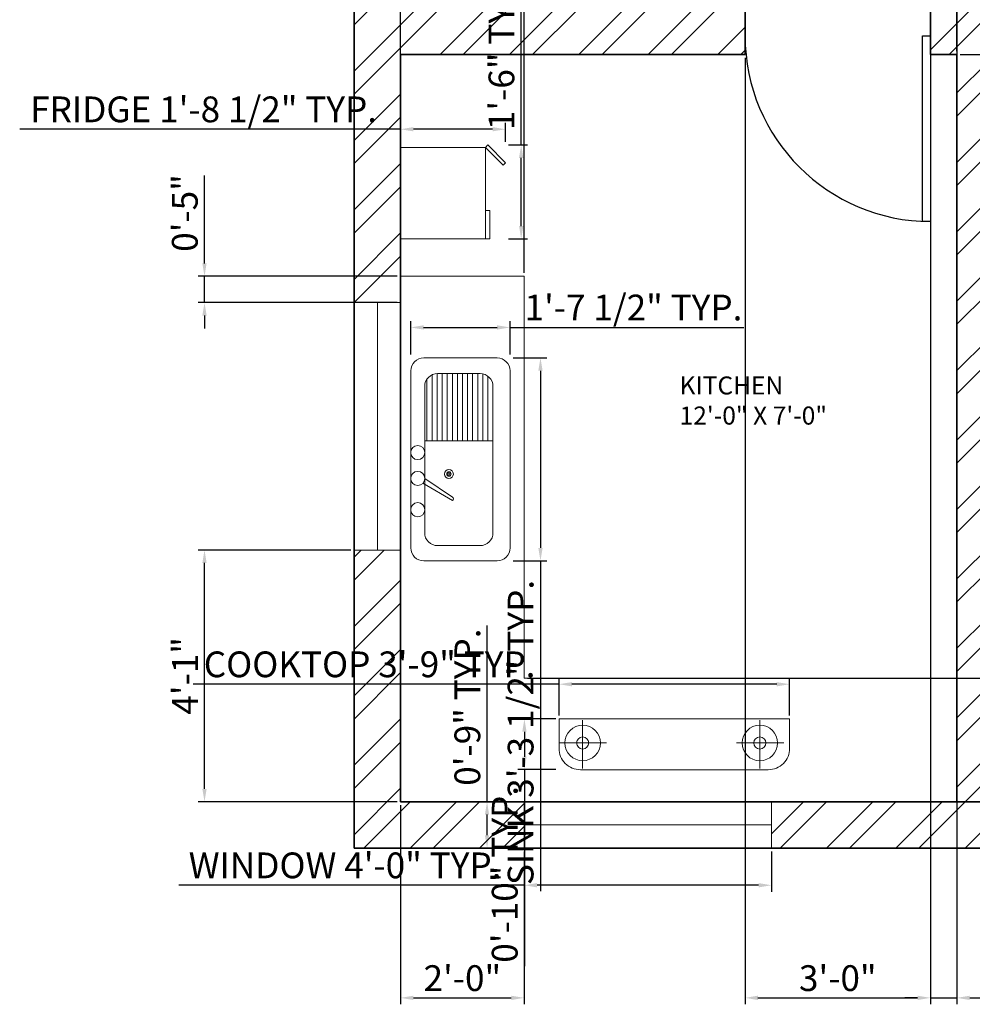
# Model space of a CAD drawing. Units: inches. Extents: x 28986 to 29505, y -162 to 451.
# Tile 1 of 6: x 28986 to 29171, y -159 to 32. Entities that reach past the tile are written whole.
import ezdxf

# ---------------------------------------------------------------- set-up
doc = ezdxf.new("R2010")
doc.units = ezdxf.units.IN
doc.layers.get('Defpoints').update_dxf_attribs({"color": 120})
doc.layers.add('A-ANNO-DIMS', color=9, linetype='Continuous', lineweight=18, true_color=0xafd9aa)
doc.layers.add('A-FLOR-CASE', color=32, linetype='Continuous', lineweight=18, true_color=0xcd6928)
for name, color, linetype, lineweight in [('A-AREA-IDEN', 6, 'Continuous', 18), ('A-EQPM', 8, 'Continuous', 18), ('A-FLOR-FIXT', 9, 'Continuous', 18), ('A-GLAZ', 4, 'Continuous', 18), ('A-WALL', 7, 'Continuous', 35), ('A-WALL-PATT', 1, 'Continuous', 13), ('DOOR', 2, 'Continuous', 25)]:
    doc.layers.add(name, color=color, linetype=linetype, lineweight=lineweight)
doc.styles.get("Standard").update_dxf_attribs({"font": 'arial.ttf'})
doc.dimstyles.new('ISO-25', dxfattribs={"dimtxt": 5, "dimasz": 2.5, "dimexe": 1.25, "dimexo": 0.625, "dimtad": 1, "dimdec": 0, "dimlunit": 3, "dimtxsty": 'Standard', "dimcen": 2.5, "dimadec": 0, "dimazin": 0, "dimtfac": 1, "dimtdec": 0, "dimtmove": 0, "dimatfit": 3, "dimfxl": 1, "dimarcsym": 0})

# ---------------------------------------------------------------- blocks, each defined once
blk = doc.blocks.new('*U7')
for p, q in [((-40, 0), (-40, 6)), ((0, 0), (0, 6))]:
    blk.add_line(p, q)
blk.add_lwpolyline([(0, 0), (0, -40), (-1.75, -40), (-1.75, 0)], close=True)
blk.add_arc((0, 0), 40, 180, 270)
blk = doc.blocks.new('FRIDGE')
for points in [[(0, 16.47), (17.77, 16.47), (17.77, 0), (0, 0)], [(0, 0), (5.53, 0), (5.53, -0.88), (0, -0.88)], [(18.23, -0.47), (17.77, 0), (14.32, -3.43), (14.79, -3.9)]]:
    blk.add_lwpolyline(points, close=True)
blk = doc.blocks.new('sink')
for p, q in [((-11.38, 27.19), (-5.63, 30.57)), ((-11.01, 26.26), (-5.62, 29.92)), ((-11.03, 19), (2.23, 19)), ((-10.58, 19), (-10.58, 7)), ((-9.6, 19), (-9.6, 6.16)), ((-8.61, 19), (-8.61, 5.92)), ((-7.63, 19), (-7.63, 5.92)), ((-6.64, 19), (-6.64, 5.92)), ((-5.66, 19), (-5.66, 5.92)), ((-4.67, 19), (-4.67, 5.92)), ((-3.69, 19), (-3.69, 5.92)), ((-2.7, 19), (-2.7, 5.92)), ((-1.72, 19), (-1.72, 5.92)), ((-0.73, 19), (-0.73, 5.92)), ((0.25, 19), (0.25, 5.98)), ((1.23, 19), (1.23, 6.43))]:
    blk.add_line(p, q)
for points in [[(-11.21, 42.26), (3.04, 42.26, -0.414214), (5.54, 39.76), (5.54, 5.38, -0.414214), (3.04, 2.88), (-11.21, 2.88, -0.414214), (-13.71, 5.38), (-13.71, 39.76, -0.414214)], [(-8.53, 39.31), (-0.27, 39.31, -0.414214), (2.23, 36.81), (2.23, 8.42, -0.414214), (-0.27, 5.92), (-8.53, 5.92, -0.414214), (-11.03, 8.42), (-11.03, 36.81, -0.414214)]]:
    blk.add_lwpolyline(points, format="xyb", close=True)
for centre, radius in [((-12.38, 32.33), 1.37), ((-12.38, 26.26), 1.37), ((-6.32, 25.41), 0.854), ((-6.32, 25.41), 0.432), ((-6.32, 25.41), 0.203), ((-12.38, 21.24), 1.37)]:
    blk.add_circle(centre, radius)
blk.add_arc((-5.86, 30.24), 0.398, 306.1138, 55.3114)
blk = doc.blocks.new('STOVE')
for p, q in [((-46.84, 5.62), (-46.82, 11.55)), ((-5.51, 5.62), (-5.49, 11.55)), ((-46.84, 5.62), (-52.42, 5.62)), ((-46.84, 5.62), (-46.84, 0.29)), ((-46.84, 5.62), (-41.4, 5.62)), ((-5.51, 5.62), (-11.1, 5.62)), ((-5.51, 5.62), (-5.51, 0.29)), ((-5.51, 5.62), (-0.08, 5.62))]:
    blk.add_line(p, q)
blk.add_lwpolyline([(-48.78, 11.85), (-5, 11.85, -0.414214), (0, 6.85), (0, 0), (-53.78, 0), (-53.78, 6.85, -0.414214)], format="xyb", close=True)
for centre, radius in [((-46.84, 5.62), 4.14), ((-5.51, 5.62), 4.14), ((-46.84, 5.62), 1.41), ((-5.51, 5.62), 1.41)]:
    blk.add_circle(centre, radius)
blk = doc.blocks.new('WIN-48IN')
for p, q in [((9, 48), (0, 48)), ((4.5, 0), (4.5, 48)), ((9, 0), (0, 0))]:
    blk.add_line(p, q)
blk = doc.blocks.new('*D37')
at = {"layer": 'A-ANNO-DIMS', "color": 0, "lineweight": -2, "transparency": 16777216}
for p, q in [((29084.16, -128.93), (29084.16, -136.75)), ((29132.16, -128.93), (29132.16, -136.75)), ((29084.16, -135.5), (29017.14, -135.5)), ((29129.66, -135.5), (29086.66, -135.5))]:
    blk.add_line(p, q, dxfattribs=at)
at = {"layer": 'A-ANNO-DIMS', "color": 0, "transparency": 16777216}
for points in [[(29086.66, -135.08), (29086.66, -135.92), (29084.16, -135.5)], [(29129.66, -135.08), (29129.66, -135.92), (29132.16, -135.5)]]:
    blk.add_solid(points, dxfattribs=at)
at = {"layer": 'Defpoints', "color": 0, "transparency": 16777216}
for p in [(29084.16, -128.3), (29132.16, -128.3), (29084.16, -135.5)]:
    blk.add_point(p, dxfattribs=at)
at = {"layer": 'A-ANNO-DIMS', "color": 0, "transparency": 16777216, "insert": (29049.4, -132.29), "char_height": 5, "attachment_point": 5}
blk.add_mtext('WINDOW 4\'-0" TYP.', dxfattribs=at)
blk = doc.blocks.new('*D38')
at = {"layer": 'A-ANNO-DIMS', "color": 0, "lineweight": -2, "transparency": 16777216}
for p, q in [((29076.96, -119.3), (29076.96, -85.07)), ((29083.53, -119.3), (29075.71, -119.3)), ((29076.96, -125.8), (29076.96, -121.8)), ((29083.53, -128.3), (29075.71, -128.3))]:
    blk.add_line(p, q, dxfattribs=at)
at = {"layer": 'A-ANNO-DIMS', "color": 0, "transparency": 16777216}
for points in [[(29076.54, -121.8), (29077.37, -121.8), (29076.96, -119.3)], [(29076.54, -125.8), (29077.37, -125.8), (29076.96, -128.3)]]:
    blk.add_solid(points, dxfattribs=at)
at = {"layer": 'Defpoints', "color": 0, "transparency": 16777216}
for p in [(29076.96, -119.3), (29084.16, -119.3), (29084.16, -128.3)]:
    blk.add_point(p, dxfattribs=at)
at = {"layer": 'A-ANNO-DIMS', "color": 0, "transparency": 16777216, "insert": (29073.78, -100.94), "char_height": 5, "attachment_point": 5, "rotation": 90}
blk.add_mtext('0\'-9" TYP.', dxfattribs=at)
blk = doc.blocks.new('*D47')
at = {"layer": 'A-ANNO-DIMS', "color": 0, "lineweight": -2, "transparency": 16777216}
for p, q in [((29082.05, -33.16), (29088.58, -33.16)), ((29087.33, -35.66), (29087.33, -70.05)), ((29082.05, -72.55), (29088.58, -72.55)), ((29087.33, -72.55), (29087.33, -136.64))]:
    blk.add_line(p, q, dxfattribs=at)
at = {"layer": 'A-ANNO-DIMS', "color": 0, "transparency": 16777216}
for points in [[(29086.91, -35.66), (29087.75, -35.66), (29087.33, -33.16)], [(29086.91, -70.05), (29087.75, -70.05), (29087.33, -72.55)]]:
    blk.add_solid(points, dxfattribs=at)
at = {"layer": 'Defpoints', "color": 0, "transparency": 16777216}
for p in [(29081.42, -33.16), (29081.42, -72.55), (29087.33, -72.55)]:
    blk.add_point(p, dxfattribs=at)
at = {"layer": 'A-ANNO-DIMS', "color": 0, "transparency": 16777216, "insert": (29084.12, -105.85), "char_height": 5, "attachment_point": 5, "rotation": 90}
blk.add_mtext('SINK 3\'-3 1/2" TYP.', dxfattribs=at)
blk = doc.blocks.new('*D48')
at = {"layer": 'A-ANNO-DIMS', "color": 0, "lineweight": -2, "transparency": 16777216}
for p, q in [((29062.13, -32.54), (29062.13, -26.01)), ((29081.42, -32.54), (29081.42, -26.01)), ((29064.63, -27.26), (29078.92, -27.26)), ((29081.42, -27.26), (29126.83, -27.26))]:
    blk.add_line(p, q, dxfattribs=at)
at = {"layer": 'A-ANNO-DIMS', "color": 0, "transparency": 16777216}
for points in [[(29064.63, -26.84), (29064.63, -27.67), (29062.13, -27.26)], [(29078.92, -26.84), (29078.92, -27.67), (29081.42, -27.26)]]:
    blk.add_solid(points, dxfattribs=at)
at = {"layer": 'Defpoints', "color": 0, "transparency": 16777216}
for p in [(29081.42, -27.26), (29062.13, -33.16), (29081.42, -33.16)]:
    blk.add_point(p, dxfattribs=at)
at = {"layer": 'A-ANNO-DIMS', "color": 0, "transparency": 16777216, "insert": (29105.38, -24.04), "char_height": 5, "attachment_point": 5}
blk.add_mtext('1\'-7 1/2" TYP.', dxfattribs=at)
blk = doc.blocks.new('*D49')
at = {"layer": 'A-ANNO-DIMS', "color": 0, "lineweight": -2, "transparency": 16777216}
for p, q in [((29090.93, -102.58), (29090.93, -95.24)), ((29135.69, -102.58), (29135.69, -95.24)), ((29090.93, -96.49), (29019.89, -96.49)), ((29133.19, -96.49), (29093.43, -96.49))]:
    blk.add_line(p, q, dxfattribs=at)
at = {"layer": 'A-ANNO-DIMS', "color": 0, "transparency": 16777216}
for points in [[(29093.43, -96.08), (29093.43, -96.91), (29090.93, -96.49)], [(29133.19, -96.08), (29133.19, -96.91), (29135.69, -96.49)]]:
    blk.add_solid(points, dxfattribs=at)
at = {"layer": 'Defpoints', "color": 0, "transparency": 16777216}
for p in [(29090.93, -96.49), (29090.93, -103.21), (29135.69, -103.21)]:
    blk.add_point(p, dxfattribs=at)
at = {"layer": 'A-ANNO-DIMS', "color": 0, "transparency": 16777216, "insert": (29054.16, -93.28), "char_height": 5, "attachment_point": 5}
blk.add_mtext('COOKTOP 3\'-9" TYP.', dxfattribs=at)
blk = doc.blocks.new('*D50')
at = {"layer": 'A-ANNO-DIMS', "color": 0, "lineweight": -2, "transparency": 16777216}
for p, q in [((29090.3, -103.21), (29082.96, -103.21)), ((29084.21, -105.71), (29084.21, -110.57)), ((29090.3, -113.07), (29082.96, -113.07)), ((29084.21, -113.07), (29084.21, -151.18))]:
    blk.add_line(p, q, dxfattribs=at)
at = {"layer": 'A-ANNO-DIMS', "color": 0, "transparency": 16777216}
for points in [[(29083.79, -105.71), (29084.63, -105.71), (29084.21, -103.21)], [(29083.79, -110.57), (29084.63, -110.57), (29084.21, -113.07)]]:
    blk.add_solid(points, dxfattribs=at)
at = {"layer": 'Defpoints', "color": 0, "transparency": 16777216}
for p in [(29090.93, -103.21), (29084.21, -113.07), (29090.93, -113.07)]:
    blk.add_point(p, dxfattribs=at)
at = {"layer": 'A-ANNO-DIMS', "color": 0, "transparency": 16777216, "insert": (29081.03, -133.38), "char_height": 5, "attachment_point": 5, "rotation": 90}
blk.add_mtext('0\'-10" TYP.', dxfattribs=at)
blk = doc.blocks.new('*D51')
at = {"layer": 'A-ANNO-DIMS', "color": 0, "lineweight": -2, "transparency": 16777216}
for p, q in [((29060.16, 8.77), (29060.16, 12.45)), ((29080.53, 8.77), (29080.53, 12.45)), ((29060.16, 11.2), (28986.23, 11.2)), ((29078.03, 11.2), (29062.66, 11.2))]:
    blk.add_line(p, q, dxfattribs=at)
at = {"layer": 'A-ANNO-DIMS', "color": 0, "transparency": 16777216}
for points in [[(29062.66, 11.62), (29062.66, 10.79), (29060.16, 11.2)], [(29078.03, 11.62), (29078.03, 10.79), (29080.53, 11.2)]]:
    blk.add_solid(points, dxfattribs=at)
at = {"layer": 'Defpoints', "color": 0, "transparency": 16777216}
for p in [(29060.16, 11.2), (29060.16, 8.15), (29080.53, 8.15)]:
    blk.add_point(p, dxfattribs=at)
at = {"layer": 'A-ANNO-DIMS', "color": 0, "transparency": 16777216, "insert": (29021.94, 14.41), "char_height": 5, "attachment_point": 5}
blk.add_mtext('FRIDGE 1\'-8 1/2" TYP.', dxfattribs=at)
blk = doc.blocks.new('*D52')
at = {"layer": 'A-ANNO-DIMS', "color": 0, "lineweight": -2, "transparency": 16777216}
for p, q in [((29083.58, 8.15), (29083.58, 41.9)), ((29081.15, 8.15), (29084.83, 8.15)), ((29083.58, -7.58), (29083.58, 5.65)), ((29081.15, -10.08), (29084.83, -10.08))]:
    blk.add_line(p, q, dxfattribs=at)
at = {"layer": 'A-ANNO-DIMS', "color": 0, "transparency": 16777216}
for points in [[(29083.17, 5.65), (29084, 5.65), (29083.58, 8.15)], [(29083.17, -7.58), (29084, -7.58), (29083.58, -10.08)]]:
    blk.add_solid(points, dxfattribs=at)
at = {"layer": 'Defpoints', "color": 0, "transparency": 16777216}
for p in [(29080.53, 8.15), (29083.58, 8.15), (29080.53, -10.08)]:
    blk.add_point(p, dxfattribs=at)
at = {"layer": 'A-ANNO-DIMS', "color": 0, "transparency": 16777216, "insert": (29080.4, 26.28), "char_height": 5, "attachment_point": 5, "rotation": 90}
blk.add_mtext('1\'-6" TYP.', dxfattribs=at)
blk = doc.blocks.new('*D64')
at = {"layer": 'A-ANNO-DIMS', "color": 0, "lineweight": -2, "transparency": 16777216}
for p, q in [((29060.16, 26.32), (29060.16, 442)), ((29168.16, 26.32), (29168.16, 442)), ((29165.66, 440.75), (29062.66, 440.75))]:
    blk.add_line(p, q, dxfattribs=at)
at = {"layer": 'A-ANNO-DIMS', "color": 0, "transparency": 16777216}
for points in [[(29062.66, 441.17), (29062.66, 440.33), (29060.16, 440.75)], [(29165.66, 441.17), (29165.66, 440.33), (29168.16, 440.75)]]:
    blk.add_solid(points, dxfattribs=at)
at = {"layer": 'Defpoints', "color": 0, "transparency": 16777216}
for p in [(29060.16, 440.75), (29060.16, 25.7), (29168.16, 25.7)]:
    blk.add_point(p, dxfattribs=at)
at = {"layer": 'A-ANNO-DIMS', "color": 0, "transparency": 16777216, "insert": (29114.16, 443.93), "char_height": 5, "attachment_point": 5}
blk.add_mtext('9\'-0"', dxfattribs=at)
blk = doc.blocks.new('*D65')
at = {"layer": 'A-ANNO-DIMS', "color": 0, "lineweight": -2, "transparency": 16777216}
for p, q in [((29168.78, 25.7), (29501.46, 25.7)), ((29500.21, -116.8), (29500.21, 23.2)), ((29168.78, -119.3), (29501.46, -119.3))]:
    blk.add_line(p, q, dxfattribs=at)
at = {"layer": 'A-ANNO-DIMS', "color": 0, "transparency": 16777216}
for points in [[(29499.79, 23.2), (29500.62, 23.2), (29500.21, 25.7)], [(29499.79, -116.8), (29500.62, -116.8), (29500.21, -119.3)]]:
    blk.add_solid(points, dxfattribs=at)
at = {"layer": 'Defpoints', "color": 0, "transparency": 16777216}
for p in [(29168.16, 25.7), (29500.21, 25.7), (29168.16, -119.3)]:
    blk.add_point(p, dxfattribs=at)
at = {"layer": 'A-ANNO-DIMS', "color": 0, "transparency": 16777216, "insert": (29497.07, -46.8), "char_height": 5, "attachment_point": 5, "rotation": 90}
blk.add_mtext('12\'-1"', dxfattribs=at)
blk = doc.blocks.new('*D72')
at = {"layer": 'A-ANNO-DIMS', "color": 0, "lineweight": -2, "transparency": 16777216}
for p, q in [((29050.53, -70.45), (29020.86, -70.45)), ((29022.11, -116.8), (29022.11, -72.95)), ((29059.53, -119.3), (29020.86, -119.3))]:
    blk.add_line(p, q, dxfattribs=at)
at = {"layer": 'A-ANNO-DIMS', "color": 0, "transparency": 16777216}
for points in [[(29021.69, -72.95), (29022.52, -72.95), (29022.11, -70.45)], [(29021.69, -116.8), (29022.52, -116.8), (29022.11, -119.3)]]:
    blk.add_solid(points, dxfattribs=at)
at = {"layer": 'Defpoints', "color": 0, "transparency": 16777216}
for p in [(29022.11, -70.45), (29051.16, -70.45), (29060.16, -119.3)]:
    blk.add_point(p, dxfattribs=at)
at = {"layer": 'A-ANNO-DIMS', "color": 0, "transparency": 16777216, "insert": (29018.97, -94.87), "char_height": 5, "attachment_point": 5, "rotation": 90}
blk.add_mtext('4\'-1"', dxfattribs=at)
blk = doc.blocks.new('*D73')
at = {"layer": 'A-ANNO-DIMS', "color": 0, "lineweight": -2, "transparency": 16777216}
for p, q in [((29060.16, -119.93), (29060.16, -158.6)), ((29084.16, -128.93), (29084.16, -158.6)), ((29062.66, -157.35), (29081.66, -157.35))]:
    blk.add_line(p, q, dxfattribs=at)
at = {"layer": 'A-ANNO-DIMS', "color": 0, "transparency": 16777216}
for points in [[(29062.66, -156.93), (29062.66, -157.77), (29060.16, -157.35)], [(29081.66, -156.93), (29081.66, -157.77), (29084.16, -157.35)]]:
    blk.add_solid(points, dxfattribs=at)
at = {"layer": 'Defpoints', "color": 0, "transparency": 16777216}
for p in [(29060.16, -119.3), (29084.16, -128.3), (29084.16, -157.35)]:
    blk.add_point(p, dxfattribs=at)
at = {"layer": 'A-ANNO-DIMS', "color": 0, "transparency": 16777216, "insert": (29072.16, -154.17), "char_height": 5, "attachment_point": 5}
blk.add_mtext('2\'-0"', dxfattribs=at)
blk = doc.blocks.new('*D82')
at = {"layer": 'A-ANNO-DIMS', "color": 0, "lineweight": -2, "transparency": 16777216}
for p, q in [((29127.04, 25.07), (29127.04, -158.6)), ((29163.04, 25.07), (29163.04, -158.6)), ((29129.54, -157.35), (29160.54, -157.35))]:
    blk.add_line(p, q, dxfattribs=at)
at = {"layer": 'A-ANNO-DIMS', "color": 0, "transparency": 16777216}
for points in [[(29129.54, -156.93), (29129.54, -157.77), (29127.04, -157.35)], [(29160.54, -156.93), (29160.54, -157.77), (29163.04, -157.35)]]:
    blk.add_solid(points, dxfattribs=at)
at = {"layer": 'Defpoints', "color": 0, "transparency": 16777216}
for p in [(29127.04, 25.7), (29163.04, 25.7), (29163.04, -157.35)]:
    blk.add_point(p, dxfattribs=at)
at = {"layer": 'A-ANNO-DIMS', "color": 0, "transparency": 16777216, "insert": (29145.04, -154.17), "char_height": 5, "attachment_point": 5}
blk.add_mtext('3\'-0"', dxfattribs=at)
blk = doc.blocks.new('*D83')
at = {"layer": 'A-ANNO-DIMS', "color": 0, "lineweight": -2, "transparency": 16777216}
for p, q in [((29163.04, 25.07), (29163.04, -158.6)), ((29168.16, 25.07), (29168.16, -158.6)), ((29160.54, -157.35), (29158.04, -157.35)), ((29163.04, -157.35), (29168.16, -157.35)), ((29170.66, -157.35), (29187.7, -157.35))]:
    blk.add_line(p, q, dxfattribs=at)
at = {"layer": 'A-ANNO-DIMS', "color": 0, "transparency": 16777216}
for points in [[(29160.54, -156.93), (29160.54, -157.77), (29163.04, -157.35)], [(29170.66, -156.93), (29170.66, -157.77), (29168.16, -157.35)]]:
    blk.add_solid(points, dxfattribs=at)
at = {"layer": 'Defpoints', "color": 0, "transparency": 16777216}
for p in [(29163.04, 25.7), (29168.16, 25.7), (29168.16, -157.35)]:
    blk.add_point(p, dxfattribs=at)
at = {"layer": 'A-ANNO-DIMS', "color": 0, "transparency": 16777216, "insert": (29180.43, -154.17), "char_height": 5, "attachment_point": 5}
blk.add_mtext('0\'-5"', dxfattribs=at)
blk = doc.blocks.new('*D84')
at = {"layer": 'A-ANNO-DIMS', "color": 0, "lineweight": -2, "transparency": 16777216}
for p, q in [((29168.16, 162.07), (29168.16, -158.6)), ((29199.96, 162.07), (29199.96, -158.6)), ((29170.66, -157.35), (29197.46, -157.35))]:
    blk.add_line(p, q, dxfattribs=at)
at = {"layer": 'A-ANNO-DIMS', "color": 0, "transparency": 16777216}
for points in [[(29170.66, -156.93), (29170.66, -157.77), (29168.16, -157.35)], [(29197.46, -156.93), (29197.46, -157.77), (29199.96, -157.35)]]:
    blk.add_solid(points, dxfattribs=at)
at = {"layer": 'Defpoints', "color": 0, "transparency": 16777216}
for p in [(29168.16, 162.7), (29199.96, 162.7), (29199.96, -157.35)]:
    blk.add_point(p, dxfattribs=at)
at = {"layer": 'A-ANNO-DIMS', "color": 0, "transparency": 16777216, "insert": (29184.06, -154.17), "char_height": 5, "attachment_point": 5}
blk.add_mtext('2\'-8"', dxfattribs=at)
blk = doc.blocks.new('*D88')
at = {"layer": 'A-ANNO-DIMS', "color": 0, "lineweight": -2, "transparency": 16777216}
for p, q in [((29060.16, -16.69), (29060.16, 442)), ((29084.16, -16.69), (29084.16, 442)), ((29062.66, 440.75), (29081.66, 440.75))]:
    blk.add_line(p, q, dxfattribs=at)
at = {"layer": 'A-ANNO-DIMS', "color": 0, "transparency": 16777216}
for points in [[(29062.66, 441.17), (29062.66, 440.33), (29060.16, 440.75)], [(29081.66, 441.17), (29081.66, 440.33), (29084.16, 440.75)]]:
    blk.add_solid(points, dxfattribs=at)
at = {"layer": 'Defpoints', "color": 0, "transparency": 16777216}
for p in [(29084.16, 440.75), (29060.16, -17.32), (29084.16, -17.32)]:
    blk.add_point(p, dxfattribs=at)
at = {"layer": 'A-ANNO-DIMS', "color": 0, "transparency": 16777216, "insert": (29072.16, 443.93), "char_height": 5, "attachment_point": 5}
blk.add_mtext('2\'-0"', dxfattribs=at)
blk = doc.blocks.new('*D89')
at = {"layer": 'A-ANNO-DIMS', "color": 0, "lineweight": -2, "transparency": 16777216}
for p, q in [((29084.78, -95.3), (29501.46, -95.3)), ((29500.21, -97.8), (29500.21, -116.8)), ((29084.78, -119.3), (29501.46, -119.3))]:
    blk.add_line(p, q, dxfattribs=at)
at = {"layer": 'A-ANNO-DIMS', "color": 0, "transparency": 16777216}
for points in [[(29499.79, -97.8), (29500.62, -97.8), (29500.21, -95.3)], [(29499.79, -116.8), (29500.62, -116.8), (29500.21, -119.3)]]:
    blk.add_solid(points, dxfattribs=at)
at = {"layer": 'Defpoints', "color": 0, "transparency": 16777216}
for p in [(29084.16, -95.3), (29084.16, -119.3), (29500.21, -119.3)]:
    blk.add_point(p, dxfattribs=at)
at = {"layer": 'A-ANNO-DIMS', "color": 0, "transparency": 16777216, "insert": (29497.03, -107.3), "char_height": 5, "attachment_point": 5, "rotation": 90}
blk.add_mtext('2\'-0"', dxfattribs=at)
blk = doc.blocks.new('*D90')
at = {"layer": 'A-ANNO-DIMS', "color": 0, "lineweight": -2, "transparency": 16777216}
for p, q in [((29022.11, -14.82), (29022.11, 2.22)), ((29059.53, -17.32), (29020.86, -17.32)), ((29022.11, -22.45), (29022.11, -17.32)), ((29059.53, -22.45), (29020.86, -22.45)), ((29022.11, -24.95), (29022.11, -27.45))]:
    blk.add_line(p, q, dxfattribs=at)
at = {"layer": 'A-ANNO-DIMS', "color": 0, "transparency": 16777216}
for points in [[(29021.69, -14.82), (29022.52, -14.82), (29022.11, -17.32)], [(29021.69, -24.95), (29022.52, -24.95), (29022.11, -22.45)]]:
    blk.add_solid(points, dxfattribs=at)
at = {"layer": 'Defpoints', "color": 0, "transparency": 16777216}
for p in [(29022.11, -17.32), (29060.16, -17.32), (29060.16, -22.45)]:
    blk.add_point(p, dxfattribs=at)
at = {"layer": 'A-ANNO-DIMS', "color": 0, "transparency": 16777216, "insert": (29018.93, -5.05), "char_height": 5, "attachment_point": 5, "rotation": 90}
blk.add_mtext('0\'-5"', dxfattribs=at)

msp = doc.modelspace()

# ---------------------------------------------------------------- hatches: boundary and pattern name
at = {"layer": 'A-WALL-PATT'}
h = msp.add_hatch(dxfattribs=at)
h.set_pattern_fill('ANSI32', color=256)
h.paths.add_polyline_path([(29174.16, 34.7), (29163.04, 34.7), (29163.04, 29.3), (29163.04, 25.7), (29168.16, 25.7), (29168.16, -119.3), (29174.16, -119.3), (29174.16, -71.3), (29199.96, -71.3), (29199.96, -65.3), (29174.16, -65.3)])
h.paths.add_polyline_path([(29244.8, -65.3), (29235.96, -65.3), (29235.96, -71.3), (29244.8, -71.3)])
h.paths.add_polyline_path([(29318.16, 39.7), (29462.16, 39.7), (29462.16, 44.7), (29318.16, 44.7), (29318.16, 131.49), (29312.16, 131.49), (29312.16, -65.3), (29292.8, -65.3), (29292.8, -71.3), (29312.16, -71.3), (29312.16, -119.3), (29318.16, -119.3)])
h.paths.add_polyline_path([(29219.6, 411.7), (29051.16, 411.7), (29051.16, 368.84), (29060.16, 368.84), (29060.16, 402.7), (29204.16, 402.7), (29219.6, 402.7)])
h.paths.add_polyline_path([(29060.16, 320.84), (29051.16, 320.84), (29051.16, 231.24), (29060.16, 231.24), (29060.16, 252.7)])
h.paths.add_polyline_path([(29210.16, 265.69), (29204.76, 265.69), (29204.16, 265.69), (29204.16, 258.7), (29060.16, 258.7), (29060.16, 252.7), (29204.16, 252.7), (29204.16, 228.7), (29204.16, 168.7), (29199.96, 168.7), (29199.96, 167.47), (29199.96, 162.7), (29210.16, 162.7)])
h.paths.add_polyline_path([(29060.16, 183.24), (29051.16, 183.24), (29051.16, 162.7), (29060.16, 162.7), (29168.16, 162.7), (29168.16, 167.47), (29168.16, 168.7), (29060.16, 168.7)])
h.paths.add_polyline_path([(29060.16, 126.7), (29051.16, 126.7), (29051.16, 70.7), (29060.16, 70.7)])
h.paths.add_polyline_path([(29060.16, 25.7), (29127.04, 25.7), (29127.04, 34.7), (29060.16, 34.7), (29051.16, 34.7), (29051.16, -22.45), (29060.16, -22.45)])
h.paths.add_polyline_path([(29060.16, -70.45), (29051.16, -70.45), (29051.16, -128.3), (29084.16, -128.3), (29084.16, -119.3), (29060.16, -119.3)])
h.paths.add_polyline_path([(29174.16, -119.3), (29168.16, -119.3), (29132.16, -119.3), (29132.16, -128.3), (29174.16, -128.3)])
h.paths.add_polyline_path([(29471.16, 79.78), (29462.16, 79.78), (29462.16, -119.3), (29462.16, -128.3), (29471.16, -128.3)])
h.paths.add_polyline_path([(29462.16, 182.7), (29318.16, 182.7), (29318.16, 191.79), (29317.56, 191.79), (29312.16, 191.79), (29312.16, 167.49), (29317.56, 167.49), (29318.16, 167.49), (29318.16, 176.7), (29462.16, 176.7)])
h.paths.add_polyline_path([(29471.16, 221.37), (29462.16, 221.37), (29462.16, 135.64), (29471.16, 135.64)])
h.paths.add_polyline_path([(29471.16, 360.33), (29462.16, 360.33), (29462.16, 277.22), (29471.16, 277.22)])
h.paths.add_polyline_path([(29471.16, 411.7), (29243.6, 411.7), (29243.6, 402.7), (29462.16, 402.7), (29462.16, 384.33), (29471.16, 384.33)])
h.paths.add_polyline_path([(29348.16, 402.7), (29342.16, 402.7), (29342.16, 332.7), (29308.66, 332.7), (29308.66, 326.7), (29312.16, 326.7), (29312.16, 227.79), (29318.16, 227.79), (29318.16, 326.7), (29355.99, 326.7), (29355.99, 332.7), (29348.16, 332.7)])
h.paths.add_polyline_path([(29210.16, 326.7), (29272.66, 326.7), (29272.66, 332.1), (29272.66, 332.7), (29210.16, 332.7), (29210.16, 402.7), (29204.16, 402.7), (29204.16, 316.6), (29204.16, 301.69), (29210.16, 301.69)])

# ---------------------------------------------------------------- linework, layer by layer
at = {"layer": 'A-FLOR-CASE'}
msp.add_line((29060.16, -17.32), (29084.16, -17.32), dxfattribs=at)
for points in [[(29168.16, -119.3), (29060.16, -119.3), (29060.16, 25.7)], [(29168.16, -95.3), (29084.16, -95.3), (29084.16, -17.32)]]:
    msp.add_lwpolyline(points, dxfattribs=at)
at = {"layer": 'A-WALL'}
for p, q in [((29051.16, 411.7), (29051.16, -128.3)), ((29127.04, 25.7), (29127.04, 34.7)), ((29163.04, 25.7), (29163.04, 34.7)), ((29060.16, 25.7), (29060.16, -119.3)), ((29060.16, -119.3), (29318.16, -119.3)), ((29051.16, -128.3), (29318.16, -128.3))]:
    msp.add_line(p, q, dxfattribs=at)
for points in [[(29060.16, 25.7), (29127.04, 25.7)], [(29060.16, 25.7), (29060.16, -119.3)], [(29163.04, 25.7), (29168.16, 25.7)], [(29168.16, 25.7), (29168.16, -119.3)], [(29060.16, -119.3), (29168.16, -119.3)]]:
    msp.add_lwpolyline(points, dxfattribs=at)

# ---------------------------------------------------------------- block references
at = {"layer": 'A-EQPM', "rotation": 90}
msp.add_blockref('FRIDGE', (29076.63, -10.08), dxfattribs=at)
at = {"layer": 'A-EQPM', "xscale": 0.8324369141255479, "yscale": 0.8324369141255479, "zscale": 0.8324369141255479, "rotation": 180}
msp.add_blockref('STOVE', (29090.93, -103.21), dxfattribs=at)
at = {"layer": 'A-FLOR-FIXT', "xscale": -1, "rotation": 180}
msp.add_blockref('sink', (29075.88, -30.29), dxfattribs=at)
at = {"layer": 'A-GLAZ'}
msp.add_blockref('WIN-48IN', (29051.16, -70.45), dxfattribs=at)
at = {"layer": 'A-GLAZ', "rotation": 89.99999999999999}
msp.add_blockref('WIN-48IN', (29132.16, -128.3), dxfattribs=at)
at = {"layer": 'DOOR', "xscale": 0.8999999999999752, "yscale": 0.8999999999999752, "zscale": 0.8999999999999752}
msp.add_blockref('*U7', (29163.04, 29.3), dxfattribs=at)

# ---------------------------------------------------------------- texts
at = {"layer": 'A-AREA-IDEN', "insert": (29114.33, -36.77), "char_height": 3.5, "attachment_point": 1}
msp.add_mtext_dynamic_manual_height_columns('KITCHEN\\P12\'-0" X 7\'-0"', width=65.867, gutter_width=12.5, heights=[0], dxfattribs=at)

# ---------------------------------------------------------------- dimensions: what is measured, and where the dimension line sits
at = {"layer": 'A-ANNO-DIMS'}
for base, p1, p2, picture, middle in [((29060.16, 440.75), (29168.16, 25.7), (29060.16, 25.7), '*D64', (29114.16, 443.93)), ((29084.16, 440.75), (29060.16, -17.32), (29084.16, -17.32), '*D88', (29072.16, 443.93)), ((29199.96, -157.35), (29168.16, 162.7), (29199.96, 162.7), '*D84', (29184.06, -154.17)), ((29163.04, -157.35), (29127.04, 25.7), (29163.04, 25.7), '*D82', (29145.04, -154.17)), ((29168.16, -157.35), (29163.04, 25.7), (29168.16, 25.7), '*D83', (29180.43, -154.17)), ((29084.16, -157.35), (29060.16, -119.3), (29084.16, -128.3), '*D73', (29072.16, -154.17))]:
    dim = msp.add_linear_dim(base=base, p1=p1, p2=p2, dimstyle='ISO-25', override={"dimdec": 1, "dimlfac": 1, "dimrnd": 0, "dimzin": 1, "dimdsep": 46, "dimlunit": 4, "dimfrac": 2}, dxfattribs=at)
    dim.commit()
    dim.dimension.update_dxf_attribs({"geometry": picture, "text_midpoint": middle})
for base, p1, p2, angle, text, picture, middle in [((29083.58, 8.15), (29080.53, -10.08), (29080.53, 8.15), 90, '<> TYP.', '*D52', (29080.4, 26.28)), ((29060.16, 11.2), (29080.53, 8.15), (29060.16, 8.15), 180, 'FRIDGE <> TYP.', '*D51', (29021.94, 14.41)), ((29087.33, -72.55), (29081.42, -33.16), (29081.42, -72.55), 270, 'SINK <> TYP.', '*D47', (29084.12, -105.85)), ((29090.93, -96.49), (29135.69, -103.21), (29090.93, -103.21), 180, 'COOKTOP <> TYP.', '*D49', (29054.16, -93.28)), ((29076.96, -119.3), (29084.16, -128.3), (29084.16, -119.3), 90, '<> TYP.', '*D38', (29073.78, -100.94)), ((29084.21, -113.07), (29090.93, -103.21), (29090.93, -113.07), 270, '<> TYP.', '*D50', (29081.03, -133.38)), ((29084.16, -135.5), (29132.16, -128.3), (29084.16, -128.3), 180, 'WINDOW <> TYP.', '*D37', (29049.4, -132.29))]:
    dim = msp.add_linear_dim(base=base, p1=p1, p2=p2, angle=angle, text=text, dimstyle='ISO-25', override={"dimdec": 1, "dimlfac": 1, "dimrnd": 0, "dimzin": 1, "dimdsep": 46, "dimlunit": 4, "dimfrac": 2}, dxfattribs=at)
    dim.commit()
    dim.dimension.update_dxf_attribs({"geometry": picture, "text_midpoint": middle})
for base, p1, p2, picture, middle in [((29500.21, 25.7), (29168.16, -119.3), (29168.16, 25.7), '*D65', (29497.07, -46.8)), ((29022.11, -17.32), (29060.16, -22.45), (29060.16, -17.32), '*D90', (29018.93, -5.05)), ((29022.1068, -70.4468), (29060.1568, -119.301), (29051.1568, -70.4467), '*D72', (29018.9716, -94.8739)), ((29500.21, -119.3), (29084.16, -95.3), (29084.16, -119.3), '*D89', (29497.03, -107.3))]:
    dim = msp.add_linear_dim(base=base, p1=p1, p2=p2, angle=90, dimstyle='ISO-25', override={"dimdec": 1, "dimlfac": 1, "dimrnd": 0, "dimzin": 1, "dimdsep": 46, "dimlunit": 4, "dimfrac": 2}, dxfattribs=at)
    dim.commit()
    dim.dimension.update_dxf_attribs({"geometry": picture, "text_midpoint": middle})
dim = msp.add_linear_dim(base=(29081.42, -27.26), p1=(29062.13, -33.16), p2=(29081.42, -33.16), text='<> TYP.', dimstyle='ISO-25', override={"dimdec": 1, "dimlfac": 1, "dimrnd": 0, "dimzin": 1, "dimdsep": 46, "dimlunit": 4, "dimfrac": 2}, dxfattribs=at)
dim.commit()
dim.dimension.update_dxf_attribs({"geometry": '*D48', "text_midpoint": (29105.38, -24.04)})

doc.saveas('drawing.dxf')
